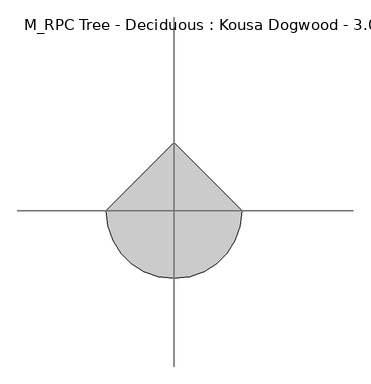
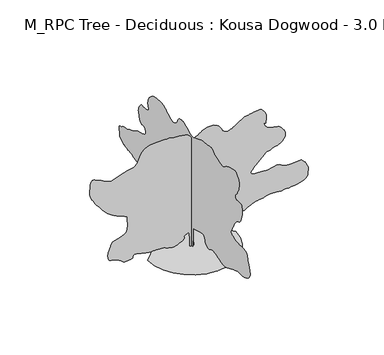
"""IFC4 building model written with IfcOpenShell, lengths in millimetres: geographic element geometry, M_RPC Tree - Deciduous : Kousa Dogwood - 3.0 Meters."""

from ifc_helpers import new_model, si_unit, origin, place, context, project, spatial, triangles, source, transform, mapped, element, save


def m_rpc_tree_deciduous_kousa_dogwood_3_0_meters_e0625334(model_context):
    return source(origin(), model_context, "Body", "Tessellation", [
        triangles([(0.0321152, 48.5607305, 0.0034119), (0.0321152, -50.059231, 0.0034119), (0.0321152, -56.2224767, 326.6823853), (0.0321152, -56.2224767, 468.4473149), (0.0321152, -179.4974194, 505.4297959), (0.0321152, -382.8998477, 573.2297636), (0.0321152, -481.5198092, 585.5572815), (0.0321152, -493.3798047, 574.9372539), (0.0321152, -505.079781, 563.9947895), (0.0321152, -516.4547771, 552.4022922), (0.0321152, -527.3447737, 539.8422667), (0.0321152, -537.5872808, 525.9872984), (0.0321152, -547.022279, 510.5148053), (0.0321152, -555.4847712, 493.1023144), (0.0321152, -561.4697619, 475.007307), (0.0321152, -564.8647582, 457.7723125), (0.0321152, -567.614772, 441.509824), (0.0321152, -571.6572578, 426.3248134), (0.0321152, -578.9372641, 412.3273393), (0.0321152, -591.3897743, 399.6223372), (0.0321152, -610.9597281, 388.3173586), (0.0321152, -633.9972754, 377.894848), (0.0321152, -655.6322193, 368.3348574), (0.0321152, -675.9747276, 360.4998705), (0.0321152, -695.1297358, 355.2548418), (0.0321152, -713.2071934, 353.4573498), (0.0321152, -730.3171955, 355.9723489), (0.0321152, -746.5597361, 363.6648663), (0.0321152, -762.949724, 373.6898357), (0.0321152, -780.3097109, 382.7473497), (0.0321152, -798.4772066, 390.9973549), (0.0321152, -817.2921919, 398.597327), (0.0321152, -836.5896332, 405.7148432), (0.0321152, -856.2146708, 412.5073428), (0.0321152, -875.999655, 419.137316), (0.0321152, -993.1095852, 400.6448401), (0.0321152, -1024.8096125, 390.0973372), (0.0321152, -1056.5095671, 379.6573494), (0.0321152, -1088.2070509, 369.4323558), (0.0321152, -1119.9070782, 359.5298716), (0.0321152, -1151.6070328, 350.0598464), (0.0321152, -1183.3045166, 341.1298682), (0.0321152, -1215.0045439, 332.8448725), (0.0321152, -1247.7819763, 324.7573574), (0.0321152, -1282.4994793, 317.2098893), (0.0321152, -1318.8344707, 311.4973746), (0.0321152, -1356.4644413, 308.9098872), (0.0321152, -1395.0644108, 310.7423698), (0.0321152, -1434.3118698, 318.2898743), (0.0321152, -1473.8818382, 332.8448725), (0.0321152, -1769.7418316, 456.1198334), (0.0321152, -1791.6092468, 465.9673064), (0.0321152, -1811.1067486, 474.5198004), (0.0321152, -1830.3892925, 481.9973236), (0.0321152, -1851.611689, 488.6098197), (0.0321152, -1876.9318005, 494.5747899), (0.0321152, -1908.5067627, 500.1098082), (0.0321152, -1948.4892059, 505.4297959), (0.0321152, -1993.2716469, 509.077284), (0.0321152, -2037.2967213, 510.4597941), (0.0321152, -2079.8141842, 511.0898066), (0.0321152, -2120.0666691, 512.4747874), (0.0321152, -2157.3016056, 516.1222755), (0.0321152, -2190.7616272, 523.5422805), (0.0321152, -2219.6915474, 536.2472826), (0.0321152, -2247.0266521, 550.8047879), (0.0321152, -2275.3291397, 563.6347824), (0.0321152, -2303.3066471, 576.0347523), (0.0321152, -2329.6691368, 589.2947714), (0.0321152, -2353.1216297, 604.7147604), (0.0321152, -2372.3665306, 623.5822861), (0.0321152, -2386.1140926, 647.1947256), (0.0321152, -2397.2190834, 669.6572353), (0.0321152, -2408.5415028, 686.5147093), (0.0321152, -2418.7840462, 701.2122133), (0.0321152, -2426.65406, 717.2072399), (0.0321152, -2430.8590359, 737.9447096), (0.0321152, -2430.1039948, 766.8771732), (0.0321152, -2423.0965736, 807.4521675), (0.0321152, -2412.5114639, 849.5371714), (0.0321152, -2401.8190933, 882.9996637), (0.0321152, -2390.9114742, 911.2846378), (0.0321152, -2379.6814911, 937.8421011), (0.0321152, -2368.0191216, 966.1271479), (0.0321152, -2355.8165234, 999.5895676), (0.0321152, -2342.9690517, 1041.6745714), (0.0321152, -2331.7716248, 1086.8520464), (0.0321152, -2322.0866055, 1126.8520758), (0.0321152, -2310.1366081, 1161.0320389), (0.0321152, -2292.1490433, 1188.7420481), (0.0321152, -2264.3491413, 1209.3345411), (0.0321152, -2222.9641674, 1222.1644993), (0.0321152, -2164.2192066, 1226.5870491), (0.0321152, -2098.4666794, 1226.6770145), (0.0321152, -2038.2142525, 1227.3044472), (0.0321152, -1982.9192265, 1229.0120464), (0.0321152, -1932.0467503, 1232.3369888), (0.0321152, -1885.0542698, 1237.8170322), (0.0321152, -1841.4043179, 1245.9944401), (0.0321152, -1800.5592819, 1257.4044994), (0.0321152, -1760.9542866, 1269.0494282), (0.0321152, -1722.9643089, 1278.862056), (0.0321152, -1688.9643494, 1288.7794739), (0.0321152, -1661.3267921, 1300.7495281), (0.0321152, -1642.4218414, 1316.7069843), (0.0321152, -1634.6243523, 1338.5944565), (0.0321152, -1640.3019127, 1368.3519424), (0.0321152, -1650.8868771, 1395.324424), (0.0321152, -1657.8043327, 1411.2994663), (0.0321152, -1663.4292801, 1421.8844307), (0.0321152, -1670.131778, 1432.6844982), (0.0321152, -1680.2843559, 1449.3068848), (0.0321152, -1696.261869, 1477.3593876), (0.0321152, -1720.43176, 1522.4468971), (0.0321152, -1744.7792564, 1570.2993542), (0.0321152, -1762.0142509, 1605.6469059), (0.0321152, -1775.5817368, 1632.5843605), (0.0321152, -1788.931794, 1655.2092876), (0.0321152, -1805.5192989, 1677.6167862), (0.0321152, -1828.7892448, 1703.9067513), (0.0321152, -1862.1967987, 1738.1767525), (0.0321152, -1899.9867886, 1769.4617615), (0.0321152, -1934.3291691, 1788.456823), (0.0321152, -1965.5416534, 1801.7368263), (0.0321152, -1993.9516926, 1815.879277), (0.0321152, -2019.8841213, 1837.4618259), (0.0321152, -2043.6591236, 1873.0592171), (0.0321152, -2065.5992088, 1929.2517174), (0.0321152, -2083.3542297, 1999.8741508), (0.0321152, -2094.4241936, 2071.5741348), (0.0321152, -2098.9166519, 2140.1491642), (0.0321152, -2096.9391563, 2201.391647), (0.0321152, -2088.6017292, 2251.0966072), (0.0321152, -2074.0091606, 2285.0590691), (0.0321152, -2053.2716183, 2299.0765274), (0.0321152, -2028.7792179, 2300.9990845), (0.0321152, -2002.9916931, 2301.6291332), (0.0321152, -1976.1267632, 2301.1790154), (0.0321152, -1948.3992405, 2299.8665955), (0.0321152, -1920.0242283, 2297.9090115), (0.0321152, -1891.2193005, 2295.5190411), (0.0321152, -1862.1967987, 2292.9116421), (0.0321152, -1846.526825, 2300.944146), (0.0321152, -1831.9342564, 2309.6241394), (0.0321152, -1819.4992596, 2319.5991119), (0.0321152, -1810.2992397, 2331.5116116), (0.0321152, -1805.4117474, 2346.0140694), (0.0321152, -1805.914333, 2363.7490334), (0.0321152, -1812.8867271, 2385.36908), (0.0321152, -1823.1842091, 2405.136478), (0.0321152, -1833.371814, 2418.9715347), (0.0321152, -1844.1018276, 2430.0064716), (0.0321152, -1856.0143272, 2441.3640633), (0.0321152, -1869.7617439, 2456.1715897), (0.0321152, -1885.9892418, 2477.5540054), (0.0321152, -1905.3416943, 2508.6489098), (0.0321152, -1927.1592579, 2549.7490173), (0.0321152, -1948.5442898, 2597.4240143), (0.0321152, -1966.7992802, 2649.1990517), (0.0321152, -1979.2367477, 2702.5739914), (0.0321152, -1983.1542412, 2755.098983), (0.0321152, -1975.8567215, 2804.2988869), (0.0321152, -1954.6517658, 2847.6488571), (0.0321152, -1927.4992081, 2886.8737885), (0.0321152, -1902.7191799, 2923.7238647), (0.0321152, -1878.1542549, 2955.8489388), (0.0321152, -1851.6491867, 2980.8488663), (0.0321152, -1821.0442234, 2996.3487923), (0.0321152, -1784.1893509, 2999.9988602), (0.0321152, -1738.9217651, 2989.4239243), (0.0321152, -1692.8293751, 2973.9487061), (0.0321152, -1653.2043228, 2962.998793), (0.0321152, -1617.4618824, 2954.3237411), (0.0321152, -1583.0144211, 2945.6486893), (0.0321152, -1547.2718353, 2934.6987762), (0.0321152, -1507.6469284, 2919.2238487), (0.0321152, -1461.554393, 2896.9487549), (0.0321152, -1417.7968895, 2870.823896), (0.0321152, -1383.95942, 2846.4239319), (0.0321152, -1355.6194347, 2825.4737572), (0.0321152, -1328.3594707, 2809.698848), (0.0321152, -1297.7569782, 2800.8238083), (0.0321152, -1259.3920235, 2800.5738235), (0.0321152, -1208.841984, 2810.6737885), (0.0321152, -1151.1220333, 2827.7739075), (0.0321152, -1095.7745396, 2846.3989334), (0.0321152, -1045.1695616, 2864.9989609), (0.0321152, -1001.6820997, 2882.1237877), (0.0321152, -967.6821402, 2896.1988007), (0.0321152, -945.5421398, 2905.7737976), (0.0321152, -937.6370991, 2909.2738747), (0.0321152, -933.2696331, 2914.6738358), (0.0321152, -920.8171228, 2928.2738777), (0.0321152, -901.2471691, 2946.1489494), (0.0321152, -875.532169, 2964.4987015), (0.0321152, -844.642194, 2979.3736656), (0.0321152, -809.5471704, 2986.9237862), (0.0321152, -771.2146992, 2983.2487198), (0.0321152, -721.277195, 2972.4237991), (0.0321152, -656.2422112, 2961.4738861), (0.0321152, -584.4172711, 2951.0739395), (0.0321152, -514.0997972, 2941.8489212), (0.0321152, -453.5948058, 2934.47379), (0.0321152, -411.2023353, 2929.5487999), (0.0321152, -395.2273293, 2927.7739082), (0.0321152, -389.2073479, 2924.6238098), (0.0321152, -372.7298653, 2916.1987427), (0.0321152, -348.1648676, 2903.9989059), (0.0321152, -317.8848845, 2889.5489159), (0.0321152, -284.2623909, 2874.3239731), (0.0321152, -249.6706434, 2859.8489845), (0.0321152, -216.4799186, 2847.6488571), (0.0321152, -182.6961704, 2835.2237434), (0.0321152, -145.4621876, 2820.7737534), (0.0321152, -105.8562113, 2806.7237389), (0.0321152, -64.9562232, 2795.5988365), (0.0321152, -23.8407913, 2789.8738953), (0.0321152, 16.4121432, 2792.023764), (0.0321152, 54.724226, 2804.4988747), (0.0321152, 95.0672077, 2825.5987495), (0.0321152, 140.4776899, 2850.2489891), (0.0321152, 188.4756686, 2875.9988708), (0.0321152, 236.5816531, 2900.3238396), (0.0321152, 282.3148899, 2920.7737541), (0.0321152, 323.1973872, 2934.8487671), (0.0321152, 356.7473742, 2940.0987373), (0.0321152, 387.7448281, 2939.8987495), (0.0321152, 421.3323492, 2938.5238335), (0.0321152, 455.5648164, 2934.7737717), (0.0321152, 488.5048116, 2927.4489281), (0.0321152, 518.2072864, 2915.3987915), (0.0321152, 542.7372934, 2897.3987274), (0.0321152, 560.1497844, 2872.298806), (0.0321152, 571.7222611, 2845.0237267), (0.0321152, 581.032267, 2820.8737473), (0.0321152, 589.584761, 2799.1989075), (0.0321152, 598.8947668, 2779.3739548), (0.0321152, 610.4672436, 2760.6989319), (0.0321152, 625.8122372, 2742.5988739), (0.0321152, 646.4422279, 2724.3738235), (0.0321152, 671.2597538, 2707.0990059), (0.0321152, 697.802247, 2692.6490158), (0.0321152, 725.529697, 2681.5238228), (0.0321152, 753.9047092, 2674.2739746), (0.0321152, 782.3872004, 2671.4488564), (0.0321152, 810.4371597, 2673.5990158), (0.0321152, 837.5196636, 2681.2238411), (0.0321152, 865.1921751, 2693.0489914), (0.0321152, 895.1296646, 2707.1490028), (0.0321152, 926.9546116, 2723.1238998), (0.0321152, 960.2896408, 2740.598996), (0.0321152, 994.7570864, 2759.2240219), (0.0321152, 1029.9771023, 2778.5990021), (0.0321152, 1065.5771095, 2798.3489594), (0.0321152, 1088.2370636, 2814.0738716), (0.0321152, 1112.1370583, 2829.173822), (0.0321152, 1138.5170614, 2842.9738518), (0.0321152, 1168.617041, 2854.848999), (0.0321152, 1203.6770376, 2864.0987251), (0.0321152, 1244.9369465, 2870.1489372), (0.0321152, 1293.6344101, 2872.298806), (0.0321152, 1349.6844772, 2871.0988792), (0.0321152, 1409.9369041, 2867.1988266), (0.0321152, 1471.0519238, 2860.1739647), (0.0321152, 1529.689333, 2849.5987381), (0.0321152, 1582.5044231, 2835.0237556), (0.0321152, 1626.1519043, 2816.0237526), (0.0321152, 1657.2943348, 2792.1737549), (0.0321152, 1679.9917866, 2768.8240173), (0.0321152, 1700.7467697, 2750.1989914), (0.0321152, 1719.8842644, 2734.2738007), (0.0321152, 1737.7292507, 2718.9988609), (0.0321152, 1754.6017673, 2702.3240067), (0.0321152, 1770.8292652, 2682.1990723), (0.0321152, 1786.7342537, 2656.5738922), (0.0321152, 1800.3918503, 2627.8738998), (0.0321152, 1809.9517319, 2599.8238678), (0.0321152, 1815.8442501, 2572.2990944), (0.0321152, 1818.5042622, 2545.2240028), (0.0321152, 1818.361829, 2518.4738914), (0.0321152, 1815.8442501, 2491.9316162), (0.0321152, 1811.3892895, 2465.4966019), (0.0321152, 1804.2368191, 2441.5614349), (0.0321152, 1794.9292477, 2421.93647), (0.0321152, 1785.8343086, 2405.6565044), (0.0321152, 1779.3293278, 2391.7465977), (0.0321152, 1777.7842186, 2379.241547), (0.0321152, 1783.5718014, 2367.1640865), (0.0321152, 1799.0618443, 2354.5490135), (0.0321152, 1819.8892067, 2343.1016018), (0.0321152, 1840.3917343, 2334.6740639), (0.0321152, 1861.0042843, 2328.511504), (0.0321152, 1882.1543015, 2323.8565556), (0.0321152, 1904.2767883, 2319.9565029), (0.0321152, 1927.7991898, 2316.0565956), (0.0321152, 1953.1541828, 2311.404118), (0.0321152, 1979.1941631, 2310.0565258), (0.0321152, 2004.4766315, 2314.2065632), (0.0321152, 2029.006675, 2320.2990692), (0.0321152, 2052.7816772, 2324.7740868), (0.0321152, 2075.7991676, 2324.0715134), (0.0321152, 2098.064233, 2314.6390949), (0.0321152, 2119.5741119, 2292.9116421), (0.0321152, 2140.2241596, 2265.2015602), (0.0321152, 2159.4692059, 2239.5416439), (0.0321152, 2176.6665573, 2214.9591328), (0.0321152, 2191.1691605, 2190.4841732), (0.0321152, 2202.326619, 2165.1441502), (0.0321152, 2209.4966755, 2137.9741516), (0.0321152, 2212.0315498, 2107.9990917), (0.0321152, 2208.9766491, 2074.5041885), (0.0321152, 2200.421648, 2037.7741631), (0.0321152, 2187.286694, 1998.3467731), (0.0321152, 2170.4840858, 1956.7642822), (0.0321152, 2150.9316456, 1913.5643028), (0.0321152, 2129.5490845, 1869.2867729), (0.0321152, 2107.2466667, 1824.469305), (0.0321152, 2067.8742153, 1829.4092651), (0.0321152, 2030.0117008, 1832.3042919), (0.0321152, 1995.1692055, 1831.0992783), (0.0321152, 1964.8517246, 1823.7492908), (0.0321152, 1940.5742821, 1808.2067802), (0.0321152, 1923.8441986, 1782.4192554), (0.0321152, 1916.1717018, 1744.3393124), (0.0321152, 1917.9141827, 1705.0943241), (0.0321152, 1927.8516575, 1675.6593475), (0.0321152, 1945.1216789, 1653.7718754), (0.0321152, 1968.8591835, 1637.1667843), (0.0321152, 1998.2041946, 1623.5818577), (0.0321152, 2032.2941196, 1610.7493561), (0.0321152, 2070.2641857, 1596.4093884), (0.0321152, 2106.9241573, 1584.1719086), (0.0321152, 2139.3791531, 1577.001852), (0.0321152, 2170.2141895, 1571.6668579), (0.0321152, 2202.0215504, 1564.9268623), (0.0321152, 2237.3865429, 1553.5518299), (0.0321152, 2278.8966545, 1534.306929), (0.0321152, 2329.1415527, 1503.9544212), (0.0321152, 2383.0889866, 1471.1769161), (0.0321152, 2433.9089951, 1445.5168545), (0.0321152, 2481.4915558, 1425.0294422), (0.0321152, 2525.7240303, 1407.7794777), (0.0321152, 2566.5238655, 1391.8218761), (0.0321152, 2603.7489189, 1375.2169304), (0.0321152, 2637.3239044, 1356.0244972), (0.0321152, 2670.0739403, 1339.9419033), (0.0321152, 2704.5488708, 1331.5145107), (0.0321152, 2740.1990204, 1327.0745201), (0.0321152, 2776.4988396, 1322.9595097), (0.0321152, 2812.8989433, 1315.5019707), (0.0321152, 2848.8737823, 1301.0370106), (0.0321152, 2883.8739716, 1275.8969753), (0.0321152, 2917.2239708, 1253.1644966), (0.0321152, 2947.6738564, 1243.4770065), (0.0321152, 2973.7987152, 1239.5070454), (0.0321152, 2994.223922, 1233.9169796), (0.0321152, 3007.5236916, 1219.3794949), (0.0321152, 3012.2986908, 1188.5620445), (0.0321152, 3007.1487144, 1134.1295385), (0.0321152, 3000.7738129, 1075.6195925), (0.0321152, 2999.8988663, 1034.3596109), (0.0321152, 3000.198848, 1005.7171005), (0.0321152, 2997.3737297, 985.049612), (0.0321152, 2987.123774, 967.7271229), (0.0321152, 2965.0989555, 949.1096546), (0.0321152, 2927.023954, 924.5646412), (0.0321152, 2887.2487656, 900.7171143), (0.0321152, 2859.3237259, 885.497113), (0.0321152, 2837.74888, 876.2071278), (0.0321152, 2817.0489807, 870.1496487), (0.0321152, 2791.6987839, 864.6321802), (0.0321152, 2756.2489128, 856.9596834), (0.0321152, 2705.1238358, 844.4346485), (0.0321152, 2648.9490669, 832.3046476), (0.0321152, 2600.4988266, 825.8897049), (0.0321152, 2557.7991074, 822.6021875), (0.0321152, 2518.7488747, 819.8521374), (0.0321152, 2481.3116249, 815.0546831), (0.0321152, 2443.4491104, 805.6196486), (0.0321152, 2403.1065147, 788.9621624), (0.0321152, 2353.7965885, 769.6621777), (0.0321152, 2293.9216095, 753.8122004), (0.0321152, 2228.7616333, 741.0897211), (0.0321152, 2163.6016571, 731.1696871), (0.0321152, 2103.7266781, 723.7297342), (0.0321152, 2054.4166065, 718.4472078), (0.0321152, 2020.9567303, 714.9972004), (0.0321152, 1997.8292175, 712.9122259), (0.0321152, 1975.5641521, 711.1496881), (0.0321152, 1953.5141899, 708.5272465), (0.0321152, 1931.0341667, 703.8547119), (0.0321152, 1907.4742676, 695.9472004), (0.0321152, 1882.1917992, 683.6197552), (0.0321152, 1854.5343304, 665.6872015), (0.0321152, 1828.8017441, 646.4947683), (0.0321152, 1807.9217686, 629.8897499), (0.0321152, 1789.194278, 613.932221), (0.0321152, 1769.9317909, 596.6822565), (0.0321152, 1747.4318562, 576.1947716), (0.0321152, 1719.0043762, 550.5347826), (0.0321152, 1681.9493706, 517.7572775), (0.0321152, 1650.1068375, 485.9673211), (0.0321152, 1634.0068027, 462.6973025), (0.0321152, 1625.991885, 445.139835), (0.0321152, 1618.4068829, 430.494835), (0.0321152, 1603.6018272, 415.9573503), (0.0321152, 1573.9143951, 398.7223557), (0.0321152, 1521.691856, 375.9923478), (0.0321152, 1461.9594555, 353.7623457), (0.0321152, 1412.9019848, 338.5423808), (0.0321152, 1371.6069763, 328.2798532), (0.0321152, 1335.1644333, 320.9298657), (0.0321152, 1300.6620335, 314.4448691), (0.0321152, 1265.1894894, 306.7698652), (0.0321152, 1225.8344788, 295.8623733), (0.0321152, 1191.2045431, 285.4223855), (0.0321152, 1167.682069, 279.5098831), (0.0321152, 1149.0120604, 276.6173816), (0.0321152, 1128.939521, 275.2323825), (0.0321152, 1101.212071, 273.8498906), (0.0321152, 1059.5745689, 270.9573891), (0.0321152, 997.7746347, 265.0448866), (0.0321152, 934.502116, 258.197394), (0.0321152, 888.5896568, 253.2924063), (0.0321152, 853.9971462, 250.0024), (0.0321152, 824.687162, 248.0084084), (0.0321152, 794.6246801, 246.9841431), (0.0321152, 757.7671915, 246.6066589), (0.0321152, 708.0797447, 246.5526469), (0.0321152, 660.1722038, 246.9301493), (0.0321152, 628.2222645, 248.0621478), (0.0321152, 605.5422535, 249.9494054), (0.0321152, 585.4522734, 252.5899056), (0.0321152, 561.2647599, 255.9873908), (0.0321152, 526.2948014, 260.1373919), (0.0321152, 473.8573045, 265.0448866), (0.0321152, 415.5448391, 270.9923979), (0.0321152, 366.6123608, 277.9098899), (0.0321152, 325.8748764, 285.2598773), (0.0321152, 292.1448858, 292.5023858), (0.0321152, 264.237396, 299.0973866), (0.0321152, 240.9663963, 304.5073761), (0.0321152, 221.1454041, 308.189873), (0.0321152, 201.9351668, 312.0898893), (0.0321152, 181.431422, 318.2523766), (0.0321152, 159.8491819, 326.3048647), (0.0321152, 137.4046944, 335.8648553), (0.0321152, 114.3129534, 346.5573712), (0.0321152, 90.7902159, 358.0023485), (0.0321152, 67.0517212, 369.8273535), (0.0321152, 30.0694877, 314.3548674), (45.1947341, 0.000153, 0.0), (-47.2612322, 0.000153, 0.0), (-47.2612322, 0.0001391, 228.0581544), (-65.7527225, 0.0001298, 369.8248464), (-189.0271793, 0.0001344, 302.0223716), (-184.0854206, 0.0001344, 286.1373855), (-181.1921742, 0.0001391, 270.0348982), (-182.3961705, 0.0001391, 253.5048934), (-189.7459218, 0.0001391, 236.3244013), (-205.2901764, 0.0001391, 218.2824067), (-231.0771562, 0.0001391, 199.1621711), (-269.154901, 0.0001437, 178.7481737), (-307.0898675, 0.0001437, 161.1374391), (-333.3798689, 0.0001437, 149.5646898), (-351.4773471, 0.0001437, 142.5206975), (-364.827368, 0.0001437, 138.4951983), (-376.8873513, 0.0001437, 135.9796996), (-391.0998559, 0.0001437, 133.4636922), (-410.9223378, 0.0001437, 129.4384473), (-433.0423176, 0.0001437, 125.9342008), (-452.7923112, 0.0001437, 125.5566984), (-471.5697988, 0.0001437, 127.6594498), (-490.7798181, 0.0001437, 131.5946929), (-511.8222836, 0.0001437, 136.716446), (-536.1022696, 0.0001437, 142.3769472), (-565.0147854, 0.0001437, 147.9294426), (-591.0347815, 0.0001437, 153.8776896), (-608.6472602, 0.0001437, 160.7961808), (-622.2672501, 0.0001437, 168.1461864), (-636.3197353, 0.0001437, 175.3879319), (-655.2247587, 0.0001437, 181.9829327), (-683.4022539, 0.0001437, 187.391923), (-725.2722273, 0.0001437, 191.0756734), (-766.9621971, 0.0001437, 193.3399248), (-795.3921478, 0.0001437, 194.8491713), (-816.1646444, 0.0001437, 195.6044304), (-834.8896643, 0.0001437, 195.6039217), (-857.1721704, 0.0001437, 194.8494256), (-888.6196695, 0.0001437, 193.3399248), (-934.8395954, 0.0001437, 191.0756734), (-986.0895922, 0.0001437, 190.8779202), (-1030.1170647, 0.0001437, 194.7774279), (-1068.7520611, 0.0001391, 201.588422), (-1103.8295712, 0.0001391, 210.1239112), (-1137.1820412, 0.0001391, 219.1989205), (-1170.6420628, 0.0001391, 227.6269126), (-1206.044553, 0.0001391, 234.2219134), (-1242.1820274, 0.0001391, 241.0504028), (-1276.2694817, 0.0001391, 249.6041503), (-1307.7719193, 0.0001391, 257.8348979), (-1336.1469315, 0.0001391, 263.6923892), (-1360.854435, 0.0001391, 265.1298923), (-1381.3594334, 0.0001391, 260.0998941), (-1397.1193726, 0.0001391, 246.5491588), (-1406.1569023, 0.0001391, 228.8306545), (-1409.8044994, 0.0001391, 212.7294208), (-1412.4819523, 0.0001391, 198.3536631), (-1418.6094852, 0.0001437, 185.8104243), (-1432.6093575, 0.0001437, 175.208437), (-1458.8994678, 0.0001437, 166.6544352), (-1501.9019302, 0.0001437, 160.2571876), (-1547.4019146, 0.0001437, 155.854186), (-1580.6118061, 0.0001437, 153.71569), (-1605.086911, 0.0001437, 154.5966864), (-1624.3868958, 0.0001437, 159.2506901), (-1642.069392, 0.0001437, 168.4334327), (-1661.6918861, 0.0001437, 182.8994283), (-1686.8143353, 0.0001391, 203.4031732), (-1714.2017624, 0.0001391, 224.6974039), (-1739.1067829, 0.0001391, 241.6791617), (-1762.8268467, 0.0001391, 255.3198988), (-1786.6567875, 0.0001391, 266.5848907), (-1811.8867882, 0.0001344, 276.4523844), (-1839.8118279, 0.0001344, 285.8848937), (-1871.7267403, 0.0001344, 295.8598844), (-1904.1442383, 0.0001344, 304.2498701), (-1932.574189, 0.0001344, 310.1623907), (-1956.796693, 0.0001344, 316.3998734), (-1976.5992634, 0.0001344, 325.7623833), (-1991.7666515, 0.0001344, 341.0548728), (-2002.0817196, 0.0001298, 365.0798598), (-2007.3292191, 0.0001298, 400.642333), (-2009.4667339, 0.0001252, 439.4223424), (-2010.0966373, 0.0001252, 472.3798147), (-2008.4617081, 0.0001252, 501.2397901), (-2003.8067596, 0.0001205, 527.7272721), (-1995.3792217, 0.0001205, 553.5672647), (-1982.4217278, 0.0001205, 580.4872785), (-1964.1817074, 0.0001159, 610.2097738), (-1949.5917549, 0.0001159, 639.8072405), (-1944.056773, 0.0001113, 665.84475), (-1941.5391941, 0.0001113, 689.2946995), (-1936.0042122, 0.0001113, 711.1297039), (-1921.4142597, 0.0001113, 732.3172188), (-1891.7266823, 0.0001066, 753.8271704), (-1840.9068192, 0.0001066, 776.6297029), (-1777.9392963, 0.0001066, 797.8696856), (-1717.5618771, 0.0001066, 815.9846409), (-1662.3568165, 0.000102, 833.8821676), (-1614.9168343, 0.000102, 854.4771315), (-1577.8268017, 0.000102, 880.6771311), (-1553.6743515, 9.74e-05, 915.3946341), (-1545.0494419, 9.74e-05, 961.542108), (-1543.4319534, 9.27e-05, 1005.7846109), (-1539.6568932, 9.27e-05, 1036.2270842), (-1535.3443657, 8.81e-05, 1057.9345528), (-1532.1093887, 8.81e-05, 1075.9745853), (-1531.5719215, 8.81e-05, 1095.4195467), (-1535.3443657, 8.81e-05, 1121.3320639), (-1545.0494419, 8.34e-05, 1158.7820309), (-1552.0394222, 8.34e-05, 1197.3995138), (-1550.4043476, 7.88e-05, 1225.451944), (-1545.8569508, 7.88e-05, 1245.9544716), (-1544.1143246, 7.88e-05, 1261.9295139), (-1550.8893471, 7.88e-05, 1276.3969448), (-1571.894315, 7.42e-05, 1292.3719872), (-1612.8493732, 7.42e-05, 1312.8745148), (-1663.2192638, 7.42e-05, 1334.9595039), (-1709.3843239, 7.42e-05, 1354.4570057), (-1752.4218132, 6.95e-05, 1372.5544476), (-1793.4117531, 6.95e-05, 1390.4344608), (-1833.431694, 6.95e-05, 1409.284473), (-1873.5591866, 6.95e-05, 1430.2919117), (-1914.8717812, 6.49e-05, 1454.6418789), (-1954.7667297, 6.49e-05, 1480.589423), (-1990.9941696, 6.49e-05, 1506.7543957), (-2025.1742054, 6.03e-05, 1534.8593662), (-2058.9217094, 6.03e-05, 1566.6293747), (-2093.8541702, 5.56e-05, 1603.7917866), (-2131.5916924, 5.56e-05, 1648.0717873), (-2173.7491482, 5.1e-05, 1701.1893299), (-2212.079076, 5.1e-05, 1748.4168251), (-2239.6291386, 4.64e-05, 1778.6042267), (-2259.95159, 4.64e-05, 1798.8768265), (-2276.6091488, 4.64e-05, 1816.3417488), (-2293.1590107, 4.17e-05, 1838.1218147), (-2313.1615688, 4.17e-05, 1871.3317062), (-2340.1690773, 3.71e-05, 1923.0842159), (-2369.5866131, 3.71e-05, 1974.4617485), (-2394.369112, 3.25e-05, 2008.0467625), (-2414.404081, 3.25e-05, 2033.2241501), (-2429.5890553, 3.25e-05, 2059.3692112), (-2439.8141579, 2.78e-05, 2095.8666927), (-2444.9714012, 2.32e-05, 2152.0940746), (-2444.9539604, 1.85e-05, 2237.4340691), (-2440.4065636, 1.39e-05, 2329.0465004), (-2431.9790257, 9.3e-06, 2398.9865627), (-2419.5614697, 9.3e-06, 2448.9790054), (-2403.0464893, 4.6e-06, 2480.7488686), (-2382.3290039, 4.6e-06, 2496.024099), (-2357.2965202, 4.6e-06, 2496.5263939), (-2327.8441029, 4.6e-06, 2483.9841362), (-2296.1790298, 4.6e-06, 2467.2014397), (-2264.7315308, 4.6e-06, 2453.111602), (-2233.7165634, 9.3e-06, 2440.641433), (-2203.3466148, 9.3e-06, 2428.7090218), (-2173.8391136, 9.3e-06, 2416.2365273), (-2145.4116337, 9.3e-06, 2402.149015), (-2118.2766621, 9.3e-06, 2385.3639931), (-2092.0391647, 1.39e-05, 2368.6715527), (-2066.1266476, 1.39e-05, 2355.2116184), (-2040.4841721, 1.39e-05, 2344.4465778), (-2015.0566544, 1.39e-05, 2335.839109), (-1989.789156, 1.39e-05, 2328.8491287), (-1964.6316799, 1.39e-05, 2322.9365536), (-1939.5292877, 1.39e-05, 2317.5640617), (-1655.9942688, 9.3e-06, 2416.1840595), (-1606.9367981, 9.3e-06, 2430.3440964), (-1556.3693905, 9.3e-06, 2441.9166458), (-1506.5568787, 4.6e-06, 2452.0863739), (-1459.7619152, 4.6e-06, 2462.0439056), (-1418.2519489, 4.6e-06, 2472.9691109), (-1384.2894871, 4.6e-06, 2486.0514519), (-1360.1368916, 4.6e-06, 2502.473996), (-1342.0595066, 4.6e-06, 2521.7239838), (-1324.9519753, 0.0, 2542.47388), (-1309.029546, 0.0, 2564.7489738), (-1294.509502, 0.0, 2588.5239761), (-1281.6069466, -4.6e-06, 2613.7988869), (-1270.5394535, -4.6e-06, 2640.5989952), (-1261.5170391, -4.6e-06, 2668.899012), (-1252.17197, -9.3e-06, 2697.4990105), (-1240.346965, -9.3e-06, 2724.7737991), (-1226.5819622, -9.3e-06, 2750.2489883), (-1211.4170448, -1.39e-05, 2773.3490318), (-1195.3869913, -1.39e-05, 2793.5239632), (-1179.0345011, -1.39e-05, 2810.2488144), (-1162.8970413, -1.39e-05, 2822.9989082), (-1145.3595217, -1.39e-05, 2835.8739944), (-1123.7220343, -1.85e-05, 2852.0988762), (-1096.9120428, -1.85e-05, 2869.7239632), (-1063.8470552, -1.85e-05, 2886.8237915), (-1023.4495937, -1.85e-05, 2901.4237724), (-974.6421078, -1.85e-05, 2911.6237312), (-916.3471195, -1.85e-05, 2915.4487885), (-850.4696726, -1.85e-05, 2916.7487091), (-781.7871643, -2.32e-05, 2919.7488167), (-713.5371878, -2.32e-05, 2923.1988968), (-648.9522491, -2.32e-05, 2925.7987381), (-591.2697598, -2.32e-05, 2926.2237122), (-543.7197916, -2.32e-05, 2923.1988968), (-509.5422993, -1.85e-05, 2915.4487885), (-481.004797, -1.85e-05, 2906.6237457), (-448.8023294, -1.85e-05, 2900.6988167), (-413.797344, -1.85e-05, 2896.848761), (-376.8498536, -1.85e-05, 2894.1739243), (-338.824849, -1.85e-05, 2891.823777), (-300.5848866, -1.85e-05, 2888.923954), (-262.9923956, -1.85e-05, 2884.6239258), (-225.8116528, -1.85e-05, 2879.5489449), (-188.9551815, -1.85e-05, 2874.2739761), (-153.5001872, -1.85e-05, 2867.79879), (-120.5252014, -1.85e-05, 2859.173735), (-91.1082107, -1.85e-05, 2847.4238708), (-66.327474, -1.39e-05, 2831.5739662), (-47.2612322, -1.39e-05, 2810.6737885), (-31.5194878, -1.39e-05, 2787.7240265), (-16.4247435, -1.39e-05, 2766.8488472), (-2.6237239, -9.3e-06, 2748.5488014), (9.2364712, -9.3e-06, 2733.3988541), (18.5090174, -9.3e-06, 2721.8989746), (24.5469392, -9.3e-06, 2714.5988388), (26.7032393, -9.3e-06, 2712.0489944), (32.9569863, -9.3e-06, 2714.1738647), (49.5612281, -9.3e-06, 2720.0987938), (73.2819686, -9.3e-06, 2729.0238304), (100.8839584, -9.3e-06, 2740.2240189), (129.1329518, -9.3e-06, 2752.9238251), (154.7941853, -1.39e-05, 2766.3738762), (174.6331814, -1.39e-05, 2779.8489258), (195.6221801, -1.39e-05, 2795.3488518), (224.805664, -1.39e-05, 2814.0988701), (259.0573887, -1.39e-05, 2834.0238167), (295.2473854, -1.85e-05, 2853.0988152), (330.2548779, -1.85e-05, 2869.2489922), (360.9473722, -1.85e-05, 2880.4488899), (384.199841, -1.85e-05, 2884.6239258), (532.1298014, -1.85e-05, 2878.4737198), (558.4372799, -1.85e-05, 2865.2489456), (584.099776, -1.85e-05, 2851.8988884), (608.4672566, -1.39e-05, 2838.3488434), (630.8922323, -1.39e-05, 2824.4738182), (650.7322277, -1.39e-05, 2810.173819), (667.3372461, -1.39e-05, 2795.3238533), (680.0597254, -1.39e-05, 2779.8489258), (690.2672419, -1.39e-05, 2763.8240318), (699.8271961, -9.3e-06, 2747.473867), (708.8472124, -9.3e-06, 2730.8490097), (717.4372404, -9.3e-06, 2713.9988754), (725.7022156, -9.3e-06, 2696.999041), (733.7547037, -4.6e-06, 2679.898922), (741.6971695, -4.6e-06, 2662.7238075), (758.8571686, -4.6e-06, 2650.9239464), (775.9646999, -4.6e-06, 2639.5990562), (792.9646797, -4.6e-06, 2629.2488159), (809.8021694, -4.6e-06, 2620.3490685), (826.4247013, -4.6e-06, 2613.3989113), (842.7771915, -4.6e-06, 2608.8738968), (858.8071724, 0.0, 2607.248996), (876.1296616, -4.6e-06, 2608.7739029), (896.2571394, -4.6e-06, 2613.2989174), (918.9721046, -4.6e-06, 2620.8490379), (944.0571287, -4.6e-06, 2631.3989754), (971.2995792, -4.6e-06, 2644.9990173), (1000.4845711, -4.6e-06, 2661.5988762), (1031.3920595, -4.6e-06, 2681.2238411), (1066.8120632, -9.3e-06, 2705.2988251), (1107.9445816, -9.3e-06, 2733.4738495), (1152.2045254, -1.39e-05, 2763.0487885), (1197.0045525, -1.39e-05, 2791.3488052), (1239.7545593, -1.39e-05, 2815.6487755), (1277.8695293, -1.39e-05, 2833.248864), (1308.7595043, -1.85e-05, 2841.4739433), (1336.0744068, -1.85e-05, 2844.673748), (1365.0069431, -1.85e-05, 2848.8237854), (1395.2869263, -1.85e-05, 2853.773774), (1426.6444599, -1.85e-05, 2859.3737228), (1458.8093571, -1.85e-05, 2865.4739319), (1491.5143375, -1.85e-05, 2871.8738319), (1524.4918304, -1.85e-05, 2878.4737198), (1554.751902, -1.85e-05, 2882.298777), (1584.3143417, -1.85e-05, 2885.2988846), (1612.4719254, -1.85e-05, 2886.7237976), (1638.5293465, -1.85e-05, 2885.6988602), (1661.7818516, -1.85e-05, 2881.4238304), (1681.5318089, -1.85e-05, 2873.1237556), (1697.0743195, -1.85e-05, 2859.9739769), (1712.241853, -1.85e-05, 2841.9739128), (1730.1042801, -1.39e-05, 2820.0737961), (1748.8292999, -1.39e-05, 2794.9488762), (1766.5843208, -1.39e-05, 2767.2488228), (1781.5342804, -9.3e-06, 2737.5988884), (1791.8493484, -9.3e-06, 2706.6490334), (1795.6943172, -4.6e-06, 2675.0489273), (1795.1568501, -4.6e-06, 2644.7990295), (1793.6467678, -4.6e-06, 2617.1239746), (1791.3268513, 0.0, 2591.5990791), (1788.3617706, 0.0, 2567.8240768), (1784.9118359, 0.0, 2545.3239967), (1781.1392464, 4.6e-06, 2523.6738647), (1777.2043121, 4.6e-06, 2502.473996), (1764.1943504, 4.6e-06, 2507.4989799), (1752.3693455, 4.6e-06, 2511.0240555), (1742.9168701, 4.6e-06, 2511.524025), (1737.0217358, 4.6e-06, 2507.4989799), (1735.871806, 4.6e-06, 2497.4440704), (1740.6517467, 4.6e-06, 2479.8340988), (1752.5492764, 4.6e-06, 2453.1665405), (1769.3142414, 9.3e-06, 2424.4140804), (1787.0518215, 9.3e-06, 2401.2689816), (1804.4642761, 9.3e-06, 2383.2990028), (1820.2592422, 1.39e-05, 2370.0716125), (1833.1442116, 1.39e-05, 2361.1590752), (1841.824205, 1.39e-05, 2356.1265335), (1845.0042435, 1.39e-05, 2354.5465427), (1974.4441624, 1.39e-05, 2323.7266216), (2073.0641602, 1.39e-05, 2305.2366165), (2122.3740864, 1.85e-05, 2280.5815807), (2149.9216782, 1.85e-05, 2248.9715916), (2176.3366356, 2.32e-05, 2217.9015404), (2200.4890858, 2.32e-05, 2187.909185), (2221.2440689, 2.32e-05, 2159.5341728), (2237.4715668, 2.78e-05, 2133.3165871), (2248.0366196, 2.78e-05, 2109.7941856), (2251.8115345, 2.78e-05, 2089.5066158), (2251.524052, 2.78e-05, 2068.1941086), (2249.5115295, 3.25e-05, 2042.0291359), (2244.0490723, 3.25e-05, 2012.1991253), (2233.4116402, 3.71e-05, 1979.8891788), (2215.8715771, 3.71e-05, 1946.2842533), (2189.7066044, 3.71e-05, 1912.5717762), (2153.1916821, 4.17e-05, 1879.9393204), (2114.681678, 4.17e-05, 1854.7792282), (2082.1016899, 4.17e-05, 1840.1892757), (2053.0791882, 4.17e-05, 1832.3893158), (2025.2442593, 4.64e-05, 1827.6092297), (1996.2217575, 4.64e-05, 1822.0742477), (1963.6442402, 4.64e-05, 1812.0117805), (1925.1342361, 4.64e-05, 1793.6467678), (1889.0317886, 4.64e-05, 1776.5918495), (1862.7418236, 4.64e-05, 1769.6742485), (1842.4892807, 4.64e-05, 1767.9317677), (1824.5017159, 4.64e-05, 1766.4042446), (1805.0042141, 4.64e-05, 1760.1318077), (1780.2218605, 5.1e-05, 1744.1567654), (1746.3842457, 5.1e-05, 1713.5167751), (1481.3444641, 6.49e-05, 1460.8044388), (1461.8818439, 6.95e-05, 1433.2019085), (1444.5244732, 6.95e-05, 1406.4095032), (1431.3694622, 6.95e-05, 1381.234441), (1424.5243858, 7.42e-05, 1358.4819054), (1426.0869358, 7.42e-05, 1338.9669628), (1438.1619255, 7.42e-05, 1323.4945061), (1462.854459, 7.42e-05, 1312.8745148), (1495.0193562, 7.42e-05, 1306.9819965), (1528.4793777, 7.42e-05, 1304.2144329), (1563.7743164, 7.42e-05, 1303.1719093), (1601.4393139, 7.42e-05, 1302.4520405), (1642.0143082, 7.42e-05, 1300.6544758), (1686.0418533, 7.42e-05, 1296.379446), (1734.0568005, 7.42e-05, 1288.219479), (1788.6517239, 7.42e-05, 1285.9745579), (1850.0367851, 7.42e-05, 1295.9120327), (1915.1967613, 7.42e-05, 1311.3469917), (1981.1091625, 7.42e-05, 1325.596994), (2044.7592018, 7.42e-05, 1331.9769825), (2103.1267147, 7.42e-05, 1323.8019001), (2153.1916821, 7.42e-05, 1294.3845097), (2211.5940765, 7.88e-05, 1263.4945347), (2290.5915802, 7.88e-05, 1251.039481), (2380.5840523, 7.88e-05, 1250.5544815), (2471.979055, 7.88e-05, 1255.569437), (2555.1739769, 7.88e-05, 1259.6120682), (2620.5990532, 7.88e-05, 1256.2144558), (2658.6240578, 7.88e-05, 1238.9095528), (2678.2990196, 7.88e-05, 1215.9270166), (2695.2738556, 8.34e-05, 1198.4420374), (2709.8738365, 8.34e-05, 1184.4069929), (2722.448941, 8.34e-05, 1171.7745518), (2733.2738617, 8.34e-05, 1158.4945484), (2742.7238663, 8.34e-05, 1142.5195787), (2751.073938, 8.81e-05, 1121.7995499), (2759.9239792, 8.81e-05, 1100.8995901), (2769.8739532, 8.81e-05, 1083.6670664), (2779.6989349, 8.81e-05, 1066.9720825), (2788.223996, 9.27e-05, 1047.6896112), (2794.2989159, 9.27e-05, 1022.6946253), (2796.6737709, 9.27e-05, 988.8570831), (2794.2239204, 9.74e-05, 943.0521029), (2791.0988205, 0.000102, 894.8196545), (2788.9739502, 0.000102, 854.5671696), (2782.7487488, 0.000102, 820.4596584), (2767.3238182, 0.0001066, 790.6646748), (2737.6988823, 0.0001066, 763.3496996), (2688.7739616, 0.0001113, 736.682214), (2615.4740753, 0.0001113, 708.8296989), (2533.8991127, 0.0001113, 685.0372559), (2461.6840439, 0.0001113, 670.1947025), (2396.1640606, 0.0001159, 661.9272566), (2334.6365662, 0.0001159, 657.8672573), (2274.3991093, 0.0001159, 655.6372335), (2212.7615925, 0.0001159, 652.8697426), (2147.0266514, 0.0001159, 647.1922548), (2085.8042255, 0.0001159, 644.2622738), (2036.1167061, 0.0001159, 648.6647667), (1992.8966698, 0.0001159, 656.4097155), (1951.0817802, 0.0001113, 663.5097181), (1905.5992367, 0.0001113, 665.9697424), (1851.3842319, 0.0001159, 659.8072552), (1783.3667267, 0.0001159, 641.0272242), (1715.8542778, 0.0001159, 620.4522446), (1663.6517956, 0.0001159, 609.257252), (1622.4442818, 0.0001159, 603.9922754), (1587.9242958, 0.0001159, 601.207271), (1555.7768394, 0.0001159, 597.4497605), (1521.6869144, 0.0001159, 589.2747508), (1481.3444641, 0.0001205, 573.2272565), (1443.3569572, 0.0001205, 555.5272831), (1416.689399, 0.0001205, 543.3247939), (1397.5668743, 0.0001205, 534.5747829), (1382.2218807, 0.0001205, 527.2247955), (1366.8744164, 0.0001205, 519.2272822), (1347.7545078, 0.0001205, 508.5348026), (1321.0869495, 0.0001252, 493.0998073), (1295.0670261, 0.0001252, 477.717316), (1277.4570545, 0.0001252, 467.4023206), (1263.8344849, 0.0001252, 460.4298174), (1249.7819996, 0.0001252, 455.0748027), (1230.8770489, 0.0001252, 449.6123091), (1202.6995537, 0.0001252, 442.3148257), (1160.8295076, 0.0001252, 431.4623268), (895.7896534, 0.0001298, 382.1523643), (840.1546772, 0.0001298, 368.7823591), (796.3796602, 0.0001298, 359.7248451), (758.9647202, 0.0001298, 354.0098597), (722.4146982, 0.0001344, 350.6673675), (681.2272413, 0.0001344, 348.7273696), (629.9047199, 0.0001344, 347.21736), (562.947288, 0.0001344, 345.1698469), (488.7672956, 0.0001344, 343.2448554), (420.0873307, 0.0001344, 342.6173501), (357.874849, 0.0001344, 343.067359), (303.0998857, 0.0001344, 344.3773444), (256.7373995, 0.0001344, 346.3373629), (219.7556634, 0.0001344, 348.7273696), (193.1239314, 0.0001344, 351.3323705), (172.5304391, 0.0001298, 355.5923575), (152.907182, 0.0001298, 362.7623414), (134.092442, 0.0001298, 372.3573589), (115.924701, 0.0001298, 383.8948451), (98.2422138, 0.0001298, 396.8873297), (80.8829718, 0.0001298, 410.8498495), (63.6857248, 0.0001298, 425.2973325), (39.0307344, 0.0001252, 505.4247817), (26.7032393, 0.0001344, 289.69489), (-1057.7445934, 0.0, 0.0031152), (-1029.7795853, -242.364912, 0.0031152), (-950.1421497, -464.9373184, 0.0031152), (-825.2021742, -661.344734, 0.0031152), (-661.344734, -825.204645, 0.0031152), (-464.9373184, -950.1421497, 0.0031152), (-242.364912, -1029.7795853, 0.0031152), (4.62e-05, -1057.7445934, 0.0031152), (242.3651482, -1029.7795853, 0.0031152), (464.9373184, -950.1421497, 0.0031152), (661.344734, -825.2021742, 0.0031152), (825.204645, -661.344734, 0.0031152), (950.1421497, -464.9373184, 0.0031152), (1029.7795853, -242.364912, 0.0031152), (1057.7445934, 9.27e-05, 0.0031152), (-0.0001387, 1057.7445934, 0.0031152)], [[451, 1, 2], [451, 2, 3], [451, 3, 4], [450, 451, 4], [316, 317, 318], [316, 318, 319], [315, 316, 319], [356, 357, 358], [355, 356, 358], [354, 355, 358], [354, 358, 359], [353, 354, 359], [353, 359, 360], [133, 134, 135], [133, 135, 136], [132, 133, 136], [132, 136, 137], [132, 137, 138], [131, 132, 138], [131, 138, 139], [131, 139, 140], [130, 131, 140], [130, 140, 141], [130, 141, 142], [129, 130, 142], [128, 129, 142], [127, 128, 142], [126, 127, 142], [125, 126, 142], [124, 125, 142], [123, 124, 142], [122, 123, 142], [122, 142, 143], [121, 122, 143], [121, 143, 144], [121, 144, 145], [120, 121, 145], [119, 120, 145], [119, 145, 146], [118, 119, 146], [315, 319, 320], [314, 315, 320], [313, 314, 320], [312, 313, 320], [311, 312, 320], [310, 311, 320], [309, 310, 320], [308, 309, 320], [307, 308, 320], [306, 307, 320], [305, 306, 320], [304, 305, 320], [304, 320, 321], [303, 304, 321], [302, 303, 321], [301, 302, 321], [300, 301, 321], [299, 300, 321], [298, 299, 321], [297, 298, 321], [296, 297, 321], [295, 296, 321], [294, 295, 321], [293, 294, 321], [292, 293, 321], [292, 321, 322], [291, 292, 322], [290, 291, 322], [289, 290, 322], [289, 322, 323], [288, 289, 323], [352, 353, 360], [352, 360, 361], [117, 118, 146], [351, 352, 361], [350, 351, 361], [349, 350, 361], [348, 349, 361], [347, 348, 361], [347, 361, 362], [347, 362, 363], [347, 363, 364], [347, 364, 365], [347, 365, 366], [347, 366, 367], [347, 367, 368], [347, 368, 369], [347, 369, 370], [347, 370, 371], [347, 371, 372], [347, 372, 373], [347, 373, 374], [346, 347, 374], [346, 374, 375], [346, 375, 376], [345, 346, 376], [345, 376, 377], [344, 345, 377], [343, 344, 377], [343, 377, 378], [342, 343, 378], [341, 342, 378], [341, 378, 379], [340, 341, 379], [340, 379, 380], [340, 380, 381], [339, 340, 381], [339, 381, 382], [339, 382, 383], [338, 339, 383], [338, 383, 384], [337, 338, 384], [337, 384, 385], [336, 337, 385], [335, 336, 385], [334, 335, 385], [333, 334, 385], [333, 385, 386], [332, 333, 386], [332, 386, 387], [332, 387, 388], [331, 332, 388], [331, 388, 389], [331, 389, 390], [330, 331, 390], [329, 330, 390], [329, 390, 391], [328, 329, 391], [328, 391, 392], [328, 392, 393], [327, 328, 393], [327, 393, 394], [327, 394, 395], [327, 395, 396], [326, 327, 396], [326, 396, 397], [326, 397, 398], [326, 398, 399], [326, 399, 400], [326, 400, 401], [326, 401, 402], [325, 326, 402], [288, 323, 324], [116, 117, 146], [116, 146, 147], [115, 116, 147], [114, 115, 147], [113, 114, 147], [112, 113, 147], [111, 112, 147], [110, 111, 147], [325, 402, 403], [204, 205, 206], [167, 168, 169], [167, 169, 170], [166, 167, 170], [165, 166, 170], [165, 170, 171], [164, 165, 171], [164, 171, 172], [163, 164, 172], [162, 163, 172], [161, 162, 172], [160, 161, 172], [159, 160, 172], [158, 159, 172], [158, 172, 173], [157, 158, 173], [157, 173, 174], [156, 157, 174], [156, 174, 175], [155, 156, 175], [155, 175, 176], [154, 155, 176], [153, 154, 176], [152, 153, 176], [152, 176, 177], [151, 152, 177], [151, 177, 178], [151, 178, 179], [150, 151, 179], [150, 179, 180], [149, 150, 180], [149, 180, 181], [148, 149, 181], [148, 181, 182], [147, 148, 182], [110, 147, 182], [110, 182, 183], [110, 183, 184], [110, 184, 185], [110, 185, 186], [109, 110, 186], [109, 186, 187], [108, 109, 187], [108, 187, 188], [107, 108, 188], [107, 188, 189], [107, 189, 190], [107, 190, 191], [106, 107, 191], [89, 90, 91], [89, 91, 92], [88, 89, 92], [88, 92, 93], [87, 88, 93], [87, 93, 94], [86, 87, 94], [86, 94, 95], [85, 86, 95], [84, 85, 95], [84, 95, 96], [83, 84, 96], [83, 96, 97], [82, 83, 97], [81, 82, 97], [80, 81, 97], [79, 80, 97], [78, 79, 97], [77, 78, 97], [76, 77, 97], [75, 76, 97], [74, 75, 97], [73, 74, 97], [72, 73, 97], [71, 72, 97], [70, 71, 97], [69, 70, 97], [68, 69, 97], [67, 68, 97], [66, 67, 97], [65, 66, 97], [64, 65, 97], [63, 64, 97], [62, 63, 97], [61, 62, 97], [60, 61, 97], [59, 60, 97], [58, 59, 97], [57, 58, 97], [57, 97, 98], [56, 57, 98], [56, 98, 99], [55, 56, 99], [55, 99, 100], [54, 55, 100], [54, 100, 101], [53, 54, 101], [53, 101, 102], [52, 53, 102], [51, 52, 102], [50, 51, 102], [50, 102, 103], [50, 103, 104], [50, 104, 105], [49, 50, 105], [48, 49, 105], [47, 48, 105], [46, 47, 105], [45, 46, 105], [44, 45, 105], [43, 44, 105], [42, 43, 105], [41, 42, 105], [40, 41, 105], [39, 40, 105], [38, 39, 105], [37, 38, 105], [36, 37, 105], [35, 36, 105], [35, 105, 106], [35, 106, 191], [34, 35, 191], [33, 34, 191], [32, 33, 191], [31, 32, 191], [30, 31, 191], [29, 30, 191], [28, 29, 191], [27, 28, 191], [26, 27, 191], [25, 26, 191], [24, 25, 191], [23, 24, 191], [22, 23, 191], [21, 22, 191], [20, 21, 191], [19, 20, 191], [18, 19, 191], [17, 18, 191], [16, 17, 191], [15, 16, 191], [14, 15, 191], [13, 14, 191], [12, 13, 191], [11, 12, 191], [10, 11, 191], [9, 10, 191], [8, 9, 191], [7, 8, 191], [6, 7, 191], [5, 6, 191], [5, 191, 192], [5, 192, 193], [5, 193, 194], [5, 194, 195], [5, 195, 196], [5, 196, 197], [5, 197, 198], [5, 198, 199], [5, 199, 200], [5, 200, 201], [5, 201, 202], [5, 202, 203], [5, 203, 204], [5, 204, 206], [5, 206, 207], [5, 207, 208], [5, 208, 209], [5, 209, 210], [5, 210, 211], [5, 211, 212], [5, 212, 213], [5, 213, 214], [5, 214, 215], [5, 215, 216], [5, 216, 217], [5, 217, 218], [4, 5, 218], [4, 218, 219], [4, 219, 220], [4, 220, 221], [4, 221, 222], [4, 222, 223], [4, 223, 224], [4, 224, 225], [4, 225, 226], [4, 226, 227], [4, 227, 228], [4, 228, 229], [4, 229, 230], [4, 230, 231], [4, 231, 232], [4, 232, 233], [4, 233, 234], [4, 234, 235], [4, 235, 236], [4, 236, 237], [4, 237, 238], [4, 238, 239], [4, 239, 240], [4, 240, 241], [4, 241, 242], [4, 242, 243], [4, 243, 244], [4, 244, 245], [450, 4, 245], [449, 450, 245], [448, 449, 245], [447, 448, 245], [446, 447, 245], [445, 446, 245], [444, 445, 245], [443, 444, 245], [442, 443, 245], [441, 442, 245], [440, 441, 245], [439, 440, 245], [438, 439, 245], [437, 438, 245], [436, 437, 245], [435, 436, 245], [434, 435, 245], [433, 434, 245], [432, 433, 245], [431, 432, 245], [430, 431, 245], [429, 430, 245], [428, 429, 245], [427, 428, 245], [426, 427, 245], [425, 426, 245], [424, 425, 245], [423, 424, 245], [422, 423, 245], [422, 245, 246], [421, 422, 246], [420, 421, 246], [419, 420, 246], [418, 419, 246], [417, 418, 246], [416, 417, 246], [415, 416, 246], [414, 415, 246], [413, 414, 246], [412, 413, 246], [411, 412, 246], [410, 411, 246], [409, 410, 246], [408, 409, 246], [407, 408, 246], [406, 407, 246], [405, 406, 246], [404, 405, 246], [403, 404, 246], [325, 403, 246], [324, 325, 246], [288, 324, 246], [288, 246, 247], [288, 247, 248], [288, 248, 249], [287, 288, 249], [287, 249, 250], [287, 250, 251], [287, 251, 252], [287, 252, 253], [287, 253, 254], [287, 254, 255], [287, 255, 256], [287, 256, 257], [287, 257, 258], [287, 258, 259], [287, 259, 260], [287, 260, 261], [287, 261, 262], [287, 262, 263], [286, 287, 263], [286, 263, 264], [286, 264, 265], [286, 265, 266], [286, 266, 267], [286, 267, 268], [286, 268, 269], [286, 269, 270], [285, 286, 270], [285, 270, 271], [285, 271, 272], [285, 272, 273], [285, 273, 274], [285, 274, 275], [285, 275, 276], [285, 276, 277], [285, 277, 278], [285, 278, 279], [285, 279, 280], [285, 280, 281], [285, 281, 282], [284, 285, 282], [284, 282, 283], [751, 752, 753], [906, 452, 453], [906, 453, 454], [906, 454, 455], [905, 906, 455], [751, 753, 754], [750, 751, 754], [750, 754, 755], [749, 750, 755], [600, 601, 602], [599, 600, 602], [599, 602, 603], [598, 599, 603], [598, 603, 604], [597, 598, 604], [597, 604, 605], [597, 605, 606], [596, 597, 606], [596, 606, 607], [596, 607, 608], [596, 608, 609], [595, 596, 609], [595, 609, 610], [595, 610, 611], [594, 595, 611], [593, 594, 611], [592, 593, 611], [591, 592, 611], [591, 611, 612], [590, 591, 612], [590, 612, 613], [589, 590, 613], [589, 613, 614], [589, 614, 615], [588, 589, 615], [588, 615, 616], [587, 588, 616], [586, 587, 616], [585, 586, 616], [584, 585, 616], [584, 616, 617], [583, 584, 617], [582, 583, 617], [581, 582, 617], [580, 581, 617], [580, 617, 618], [579, 580, 618], [578, 579, 618], [577, 578, 618], [576, 577, 618], [575, 576, 618], [574, 575, 618], [573, 574, 618], [572, 573, 618], [571, 572, 618], [570, 571, 618], [570, 618, 619], [569, 570, 619], [569, 619, 620], [569, 620, 621], [568, 569, 621], [568, 621, 622], [567, 568, 622], [567, 622, 623], [567, 623, 624], [566, 567, 624], [566, 624, 625], [566, 625, 626], [565, 566, 626], [903, 904, 905], [748, 749, 755], [565, 626, 627], [902, 903, 905], [508, 509, 510], [508, 510, 511], [507, 508, 511], [507, 511, 512], [506, 507, 512], [506, 512, 513], [505, 506, 513], [505, 513, 514], [505, 514, 515], [505, 515, 516], [505, 516, 517], [505, 517, 518], [505, 518, 519], [505, 519, 520], [505, 520, 521], [504, 505, 521], [504, 521, 522], [504, 522, 523], [747, 748, 755], [747, 755, 756], [565, 627, 628], [901, 902, 905], [900, 901, 905], [899, 900, 905], [898, 899, 905], [897, 898, 905], [896, 897, 905], [895, 896, 905], [894, 895, 905], [893, 894, 905], [892, 893, 905], [825, 826, 827], [824, 825, 827], [824, 827, 828], [823, 824, 828], [823, 828, 829], [823, 829, 830], [823, 830, 831], [823, 831, 832], [823, 832, 833], [823, 833, 834], [823, 834, 835], [822, 823, 835], [822, 835, 836], [822, 836, 837], [822, 837, 838], [822, 838, 839], [822, 839, 840], [822, 840, 841], [822, 841, 842], [822, 842, 843], [822, 843, 844], [822, 844, 845], [822, 845, 846], [822, 846, 847], [822, 847, 848], [822, 848, 849], [822, 849, 850], [821, 822, 850], [821, 850, 851], [821, 851, 852], [821, 852, 853], [820, 821, 853], [820, 853, 854], [820, 854, 855], [820, 855, 856], [820, 856, 857], [819, 820, 857], [819, 857, 858], [818, 819, 858], [817, 818, 858], [816, 817, 858], [815, 816, 858], [814, 815, 858], [814, 858, 859], [813, 814, 859], [813, 859, 860], [812, 813, 860], [812, 860, 861], [812, 861, 862], [811, 812, 862], [810, 811, 862], [810, 862, 863], [809, 810, 863], [809, 863, 864], [808, 809, 864], [808, 864, 865], [807, 808, 865], [807, 865, 866], [806, 807, 866], [806, 866, 867], [805, 806, 867], [805, 867, 868], [805, 868, 869], [804, 805, 869], [804, 869, 870], [804, 870, 871], [804, 871, 872], [804, 872, 873], [804, 873, 874], [804, 874, 875], [804, 875, 876], [804, 876, 877], [804, 877, 878], [804, 878, 879], [804, 879, 880], [804, 880, 881], [804, 881, 882], [804, 882, 883], [803, 804, 883], [803, 883, 884], [803, 884, 885], [803, 885, 886], [803, 886, 887], [803, 887, 888], [803, 888, 889], [803, 889, 890], [803, 890, 891], [802, 803, 891], [802, 891, 892], [802, 892, 905], [801, 802, 905], [800, 801, 905], [799, 800, 905], [688, 689, 690], [746, 747, 756], [905, 455, 456], [768, 769, 770], [767, 768, 770], [767, 770, 771], [767, 771, 772], [767, 772, 773], [767, 773, 774], [767, 774, 775], [767, 775, 776], [767, 776, 777], [767, 777, 778], [767, 778, 779], [767, 779, 780], [767, 780, 781], [767, 781, 782], [767, 782, 783], [767, 783, 784], [767, 784, 785], [767, 785, 786], [767, 786, 787], [767, 787, 788], [767, 788, 789], [766, 767, 789], [766, 789, 790], [766, 790, 791], [766, 791, 792], [766, 792, 793], [766, 793, 794], [766, 794, 795], [765, 766, 795], [764, 765, 795], [763, 764, 795], [763, 795, 796], [762, 763, 796], [761, 762, 796], [761, 796, 797], [761, 797, 798], [760, 761, 798], [759, 760, 798], [758, 759, 798], [757, 758, 798], [745, 746, 756], [744, 745, 756], [743, 744, 756], [742, 743, 756], [741, 742, 756], [740, 741, 756], [739, 740, 756], [738, 739, 756], [737, 738, 756], [736, 737, 756], [735, 736, 756], [734, 735, 756], [733, 734, 756], [732, 733, 756], [731, 732, 756], [730, 731, 756], [729, 730, 756], [728, 729, 756], [727, 728, 756], [726, 727, 756], [726, 756, 757], [726, 757, 798], [725, 726, 798], [724, 725, 798], [723, 724, 798], [722, 723, 798], [721, 722, 798], [720, 721, 798], [719, 720, 798], [718, 719, 798], [717, 718, 798], [716, 717, 798], [715, 716, 798], [714, 715, 798], [713, 714, 798], [712, 713, 798], [711, 712, 798], [710, 711, 798], [710, 798, 799], [710, 799, 905], [709, 710, 905], [708, 709, 905], [707, 708, 905], [706, 707, 905], [705, 706, 905], [704, 705, 905], [703, 704, 905], [702, 703, 905], [701, 702, 905], [700, 701, 905], [699, 700, 905], [698, 699, 905], [697, 698, 905], [696, 697, 905], [695, 696, 905], [694, 695, 905], [693, 694, 905], [692, 693, 905], [691, 692, 905], [690, 691, 905], [688, 690, 905], [687, 688, 905], [686, 687, 905], [685, 686, 905], [684, 685, 905], [683, 684, 905], [682, 683, 905], [681, 682, 905], [680, 681, 905], [679, 680, 905], [678, 679, 905], [677, 678, 905], [676, 677, 905], [675, 676, 905], [674, 675, 905], [674, 905, 456], [673, 674, 456], [672, 673, 456], [671, 672, 456], [670, 671, 456], [669, 670, 456], [668, 669, 456], [667, 668, 456], [666, 667, 456], [665, 666, 456], [664, 665, 456], [663, 664, 456], [662, 663, 456], [661, 662, 456], [660, 661, 456], [659, 660, 456], [658, 659, 456], [657, 658, 456], [656, 657, 456], [655, 656, 456], [654, 655, 456], [653, 654, 456], [652, 653, 456], [651, 652, 456], [650, 651, 456], [649, 650, 456], [648, 649, 456], [647, 648, 456], [646, 647, 456], [645, 646, 456], [644, 645, 456], [643, 644, 456], [642, 643, 456], [641, 642, 456], [640, 641, 456], [639, 640, 456], [638, 639, 456], [637, 638, 456], [636, 637, 456], [635, 636, 456], [634, 635, 456], [633, 634, 456], [632, 633, 456], [631, 632, 456], [630, 631, 456], [629, 630, 456], [628, 629, 456], [565, 628, 456], [564, 565, 456], [563, 564, 456], [562, 563, 456], [561, 562, 456], [560, 561, 456], [559, 560, 456], [558, 559, 456], [557, 558, 456], [556, 557, 456], [555, 556, 456], [554, 555, 456], [553, 554, 456], [552, 553, 456], [551, 552, 456], [551, 456, 457], [551, 457, 458], [551, 458, 459], [551, 459, 460], [551, 460, 461], [551, 461, 462], [551, 462, 463], [551, 463, 464], [551, 464, 465], [551, 465, 466], [551, 466, 467], [551, 467, 468], [551, 468, 469], [551, 469, 470], [551, 470, 471], [551, 471, 472], [551, 472, 473], [551, 473, 474], [551, 474, 475], [551, 475, 476], [551, 476, 477], [551, 477, 478], [551, 478, 479], [551, 479, 480], [551, 480, 481], [551, 481, 482], [551, 482, 483], [551, 483, 484], [551, 484, 485], [551, 485, 486], [551, 486, 487], [551, 487, 488], [551, 488, 489], [551, 489, 490], [551, 490, 491], [551, 491, 492], [551, 492, 493], [551, 493, 494], [551, 494, 495], [551, 495, 496], [551, 496, 497], [551, 497, 498], [551, 498, 499], [551, 499, 500], [551, 500, 501], [551, 501, 502], [551, 502, 503], [551, 503, 504], [551, 504, 523], [550, 551, 523], [549, 550, 523], [548, 549, 523], [548, 523, 524], [547, 548, 524], [547, 524, 525], [546, 547, 525], [545, 546, 525], [544, 545, 525], [543, 544, 525], [542, 543, 525], [541, 542, 525], [540, 541, 525], [540, 525, 526], [539, 540, 526], [538, 539, 526], [537, 538, 526], [536, 537, 526], [535, 536, 526], [534, 535, 526], [534, 526, 527], [533, 534, 527], [533, 527, 528], [532, 533, 528], [532, 528, 529], [531, 532, 529], [531, 529, 530], [921, 922, 907], [920, 921, 907], [920, 907, 908], [919, 920, 908], [919, 908, 909], [919, 909, 910], [918, 919, 910], [917, 918, 910], [917, 910, 911], [917, 911, 912], [917, 912, 913], [917, 913, 914], [917, 914, 915], [917, 915, 916]], closed=False),
    ])


if __name__ == "__main__":
    model = new_model("IFC4")
    model_context = context("Model", 3, world=origin())
    ifc_project = project(units=[si_unit("LENGTHUNIT", "METRE", prefix="MILLI")], contexts=[model_context])
    site = spatial("IfcSite", under=ifc_project)
    building = spatial("IfcBuilding", under=site)
    placement = place(None, origin())
    m_rpc_tree_deciduous_kousa_dogwood_3_0_meters_shape = m_rpc_tree_deciduous_kousa_dogwood_3_0_meters_e0625334(model_context)
    element("IfcGeographicElement", 1, ObjectType="M_RPC Tree - Deciduous : Kousa Dogwood - 3.0 Meters", at=placement, inside=building, context=model_context, shape_type="MappedRepresentation", body=[
        mapped(m_rpc_tree_deciduous_kousa_dogwood_3_0_meters_shape, transform((0.0, 0.0, 0.0), x_axis=(1.0, 0.0, 0.0), y_axis=(0.0, 1.0, 0.0), z_axis=(0.0, 0.0, 1.0))),
    ])
    save(model, "model.ifc")

# Revit data of these elements
# Type "M_RPC Tree - Deciduous : Kousa Dogwood - 3.0 Meters"
#   built-in parameter 1005198 = "{2, 15},{39, RPC-16-G2M3-G0FX-C7PN-N000-ST1L-LVER-AU},{1, 0},{1, 0},{2, 35},{1, 8},{5, Color},{1, 0},{1, 0},{3, 0.8},{3, 0.8},{3, 0.8},{1, 8},{7, BBoxMin},{1, 0},{1, 0},{1, 0},{1, 0},{1, 0},{1, 8},{7, BBoxMax},{1, 0},{1, 0},{1, 0},{1, 0},{1, 0},{2, 11},{9, RPCTypeId},{1, 0},{1, 0},{39, RPC-16-G2M3-G0FX-C7PN-N000-ST1L-LVER-AU},{1, 6},{14, RPCPlantHeight},{1, 0},{1, 0},{7, 9.84252},{2, 11},{7, keyword},{1, 0},{1, 0},{134, :Geometry:RPC:Kousa Dogwood:Cornus kousa:very small trees:native to eastern Asia:occasionally planted in Canada and the United States.},{2, 11},{8, category},{1, 0},{1, 0},{16, :Trees [General]},{2, 11},{12, LocalizedUID},{1, 0},{1, 0},{13, Kousa Dogwood},{2, 14},{6, Height},{1, 0},{1, 0},{7, 9.84252},{1, 2},{16, Cast Reflections},{1, 0},{1, 0},{1, 0},{1, 2},{12, Cast Shadows},{1, 0},{1, 0},{1, 1},{1, 2},{9, Lock View},{1, 0},{1, 0},{1, 0},{1, 4},{5, ViewC},{1, 0},{1, 0},{1, 0},{2, 11},{20, AdvancedUIDefinition},{1, 0},{1, 0},{0, },{2, 11},{10, AssetLibID},{1, 0},{1, 0},{36, 4D3F6E72-3F99-4203-98E9-AF80B3C7A7A4},{2, 11},{10, BaseSchema},{1, 0},{1, 0},{9, RPCSchema},{2, 11},{12, ExchangeGUID},{1, 0},{1, 0},{0, },{1, 2},{6, Hidden},{1, 0},{1, 0},{1, 0},{1, 4},{11, RPCCategory},{1, 0},{1, 0},{1, 0},{2, 11},{8, RPCImage},{1, 0},{1, 0},{0, },{1, 4},{13, SchemaVersion},{1, 0},{1, 0},{1, 4},{2, 11},{12, UIDefinition},{1, 0},{1, 0},{0, },{2, 11},{6, UIName},{1, 0},{1, 0},{39, RPC-16-G2M3-G0FX-C7PN-N000-ST1L-LVER-AU},{2, 11},{11, VersionGUID},{1, 0},{1, 0},{9, RPCSchema},{2, 11},{9, assettype},{1, 0},{1, 0},{11, RPCGeometry},{2, 11},{11, description},{1, 0},{1, 0},{0, },{2, 11},{9, localname},{1, 0},{1, 0},{3, RPC},{2, 11},{9, localtype},{1, 0},{1, 0},{3, RPC},{1, 4},{8, revision},{1, 0},{1, 0},{1, 1},{2, 11},{9, thumbnail},{1, 0},{1, 0},{0, },{1, 4},{7, version},{1, 0},{1, 0},{1, 1},{1, 2},{20, RPC_Cast Reflections},{1, 0},{1, 0},{1, 1},{1, 2},{16, RPC_Cast Shadows},{1, 0},{1, 0},{1, 1},{1, 2},{13, RPC_Lock View},{1, 0},{1, 0},{1, 0},{1, 4},{9, RPC_ViewC},{1, 0},{1, 0},{1, 0},{21, assetlibrary_base.fbx},{1, 5},"
#   built-in parameter 1005195 = "RPC-16-G2M3-G0FX-C7PN-N000-ST1L-LVER-AU"
#   Type Comments = "Kousa Dogwood"
#   Height = 9' - 10.11024"
#   Default Elevation = 0
